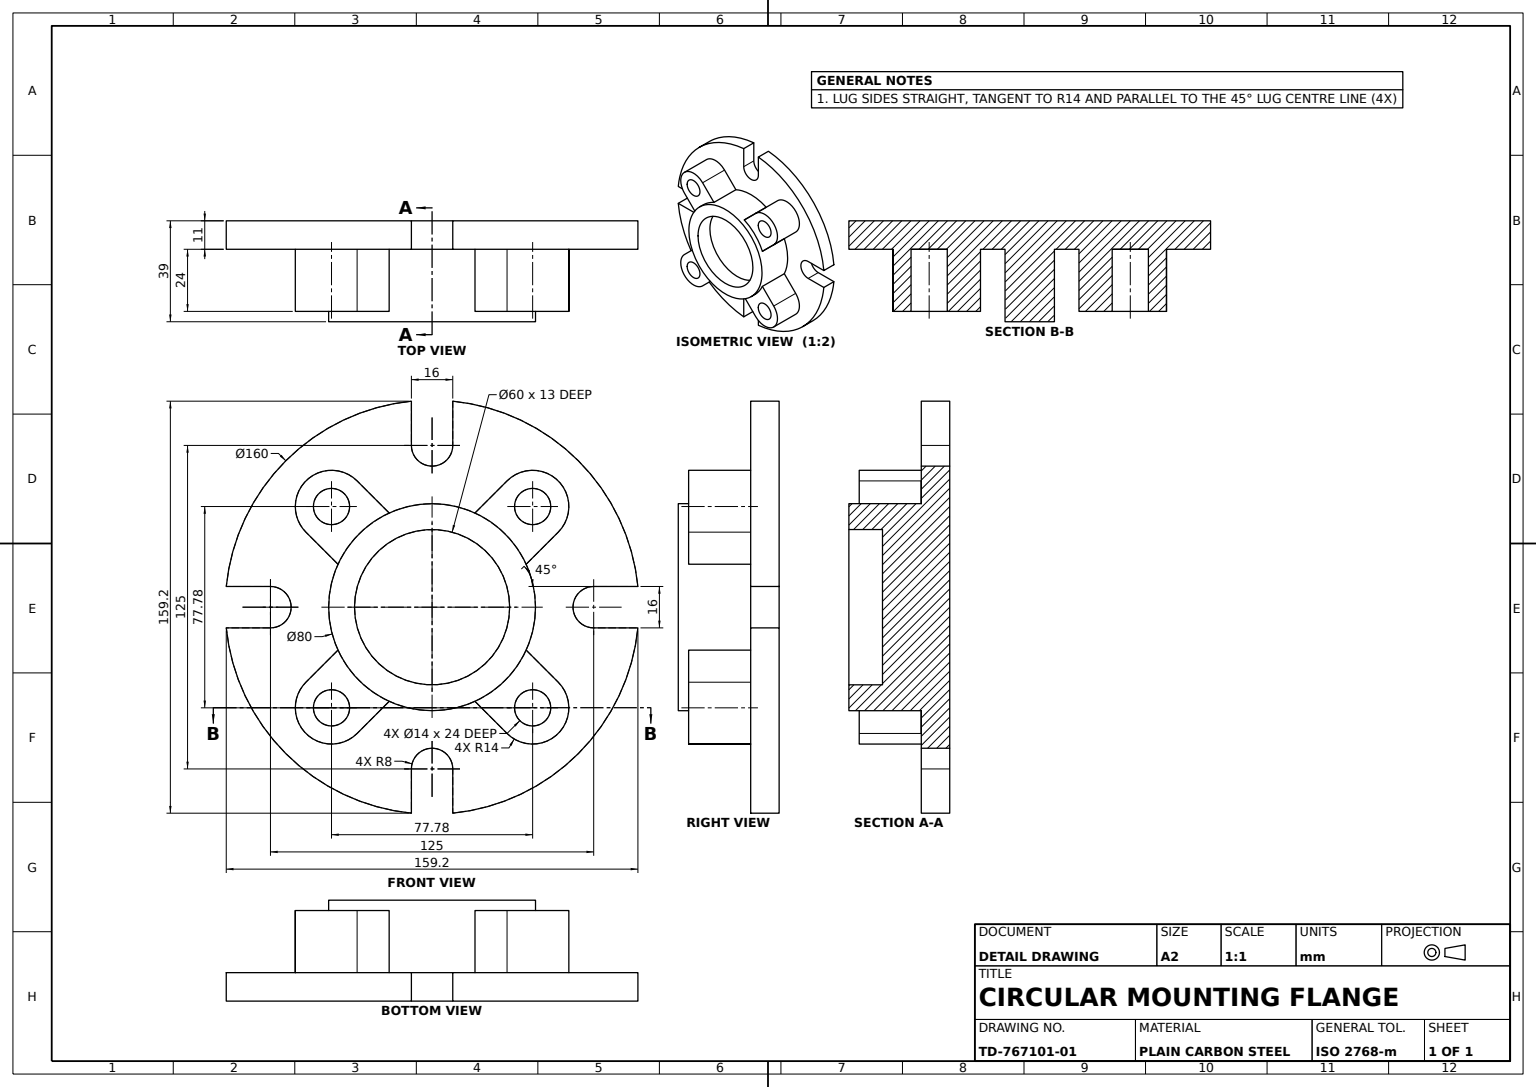
from build123d import *

# Parameters (mm, degrees)
FLANGE_DISC_SKETCH_R          = 80
FLANGE_DISC_160_DEPTH         = 11
HUB_SKETCH_R                  = 40
HUB_SKETCH_R_2                = 30
HUB_80X_60_DEPTH              = 28
ROUND_BOSS_SKETCH_R           = 30
ROUND_BOSS_15MM_DEPTH         = 15
MOUNTING_LUG_SKETCH_R         = 7
MOUNTING_LUG_DEPTH            = 24
MOUNTING_LUG_PATTERN_4X_COUNT = 4
RIM_START                     = -24
RIM_SLOT_CUT_DEPTH            = 24
RIM_SLOT_PATTERN_4X_COUNT     = 4


with BuildPart() as part:
    # Flange Disc Sketch → Flange Disc Ø160 (new body)
    with BuildSketch(Plane.XY):
        Circle(FLANGE_DISC_SKETCH_R)
    extrude(amount=FLANGE_DISC_160_DEPTH)

    # Hub Sketch → Hub Ø80xØ60 (add)
    with BuildSketch(Plane.XY.offset(11)):
        Circle(HUB_SKETCH_R)
        Circle(HUB_SKETCH_R_2, mode=Mode.SUBTRACT)
    extrude(amount=HUB_80X_60_DEPTH)

    # Round Boss Sketch → Round Boss 15mm (add)
    with BuildSketch(Plane.XY.offset(11)):
        Circle(ROUND_BOSS_SKETCH_R)
    extrude(amount=ROUND_BOSS_15MM_DEPTH)

    # Mounting Lug Sketch → Mounting Lug (add)
    with BuildSketch(Plane.XY.offset(11)):
        with BuildLine():
            Line((16.595787662, 36.394777536), (28.991378029, 48.790367902))
            ThreePointArc((28.991378029, 48.790367902), (48.790367902, 48.790367902), (48.790367902, 28.991378029))
            Line((48.790367902, 28.991378029), (36.394777536, 16.595787662))
            ThreePointArc((36.394777536, 16.595787662), (28.284271247, 28.284271247), (16.595787662, 36.394777536))
        make_face()
        with Locations((38.890872965, 38.890872965)):
            Circle(MOUNTING_LUG_SKETCH_R, mode=Mode.SUBTRACT)
    mounting_lug = extrude(amount=MOUNTING_LUG_DEPTH)

    # Mounting Lug Pattern 4x: Mounting Lug ×4 about axis
    mounting_lug_pattern_4x_axis = Axis((0, 0, 0), (0, 0, 1))
    for i in range(1, MOUNTING_LUG_PATTERN_4X_COUNT):
        add(mounting_lug.rotate(mounting_lug_pattern_4x_axis, i * 360 / MOUNTING_LUG_PATTERN_4X_COUNT))

    # Rim Slot Sketch → Rim Slot Cut (cut)
    with BuildSketch(Plane.XY.offset(11).offset(RIM_START)):
        with BuildLine():
            Line((62.5, 8), (79.598994969, 8))
            ThreePointArc((79.598994969, 8), (80, 0), (79.598994969, -8))
            Line((79.598994969, -8), (62.5, -8))
            ThreePointArc((62.5, -8), (54.5, 0), (62.5, 8))
        make_face()
    rim_slot_cut = extrude(amount=RIM_SLOT_CUT_DEPTH, mode=Mode.SUBTRACT)

    # Rim Slot Pattern 4x: Rim Slot Cut ×4 about axis
    rim_slot_pattern_4x_axis = Axis((0, 0, 0), (0, 0, 1))
    for i in range(1, RIM_SLOT_PATTERN_4X_COUNT):
        add(rim_slot_cut.rotate(rim_slot_pattern_4x_axis, i * 360 / RIM_SLOT_PATTERN_4X_COUNT), mode=Mode.SUBTRACT)


solid = part.part
